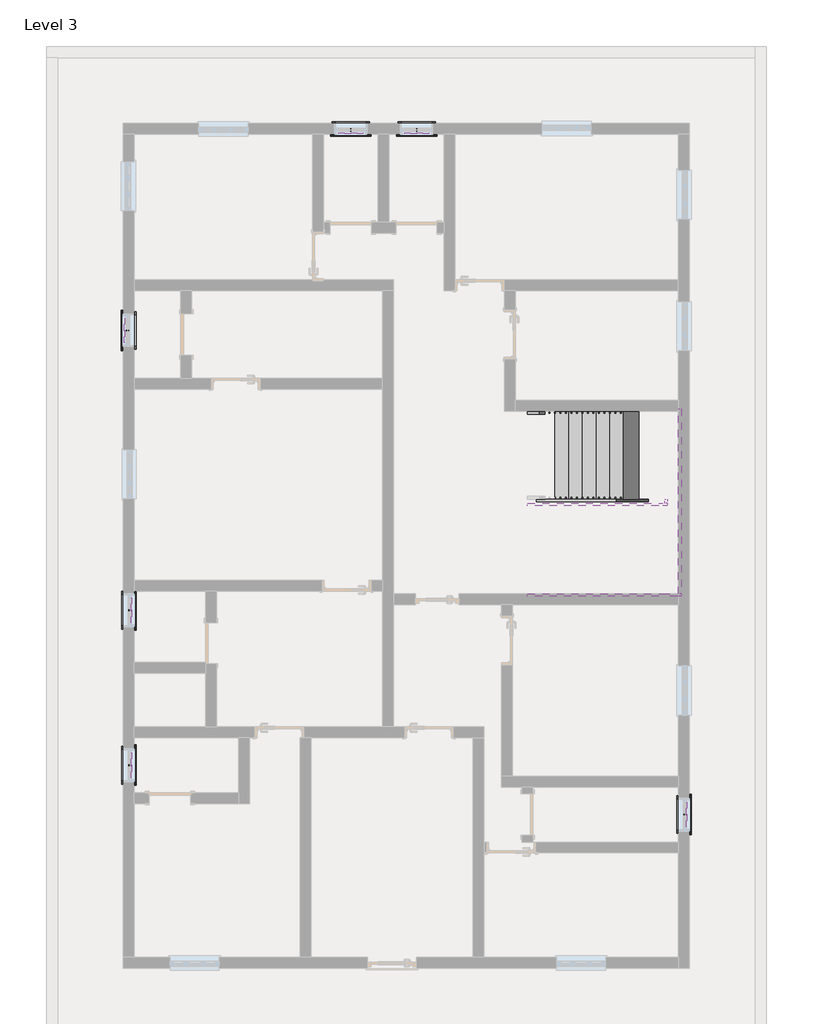
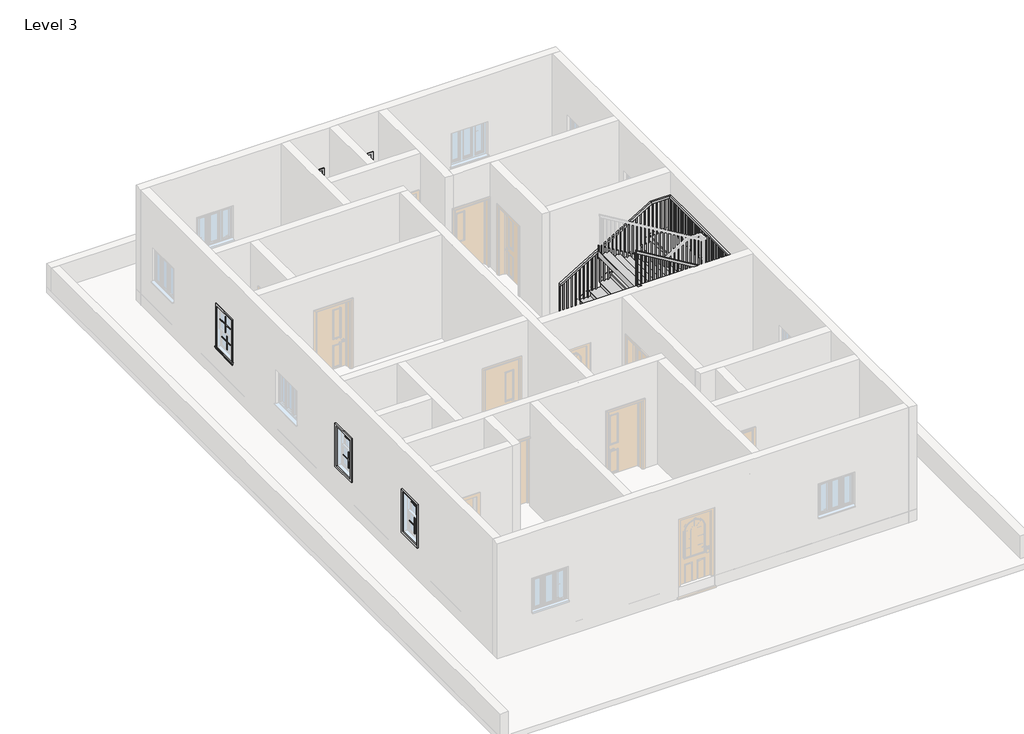
# One storey, part 3 of 3: 24 proxies, 6 members, 1 railing, 1 stair flight.
"""IFC4 building model written with IfcOpenShell, lengths in millimetres."""

from ifc_helpers import new_model, si_unit, frame, origin, place, context, project, spatial, polyline, outline, extrude, faceted_brep, transform, mapped, element, save
from components import muntin_pattern_2x2_muntin_pattern_2x2_eba6c5fb, trim_window_exterior_flat_with_sill_278e6a94, trim_window_interior_flat_picture_frame_e9fd5f45, stair_flight_8d4d0c3c

model = new_model("IFC4")

# Units and contexts
model_context = context("Model", 3, world=origin())
ifc_project = project(units=[si_unit("LENGTHUNIT", "METRE", prefix="MILLI")], contexts=[model_context])

# Site, building, storey
site = spatial("IfcSite", under=ifc_project)
building = spatial("IfcBuilding", under=site)
storey = spatial("IfcBuildingStorey", under=building, Name="Level 3", Elevation=6096.0)

# Proxies
placement = place(None, origin())
muntin_pattern_2x2_muntin_pattern_2x2_shape = muntin_pattern_2x2_muntin_pattern_2x2_eba6c5fb(model_context)
element("IfcBuildingElementProxy", 1, Name="Muntin Pattern_2x2 : Muntin Pattern_2x2", ObjectType="Muntin Pattern_2x2 : Muntin Pattern_2x2", at=placement, inside=storey, context=model_context, shape_type="MappedRepresentation", body=[
    mapped(muntin_pattern_2x2_muntin_pattern_2x2_shape, transform((-13738.8961241, 8049.5344295, 7566.025), x_axis=(0.0, -1.0, 0.0), y_axis=(1.0, 0.0, 0.0), z_axis=(0.0, 0.0, 1.0))),
])
element("IfcBuildingElementProxy", 2, Name="Muntin Pattern_2x2 : Muntin Pattern_2x2", ObjectType="Muntin Pattern_2x2 : Muntin Pattern_2x2", at=placement, inside=storey, context=model_context, shape_type="MappedRepresentation", body=[
    mapped(muntin_pattern_2x2_muntin_pattern_2x2_shape, transform((-13783.3461241, 8049.5344295, 7086.6), x_axis=(0.0, -1.0, 0.0), y_axis=(1.0, 0.0, 0.0), z_axis=(0.0, 0.0, 1.0))),
])
element("IfcBuildingElementProxy", 3, Name="Muntin Pattern_2x2 : Muntin Pattern_2x2", ObjectType="Muntin Pattern_2x2 : Muntin Pattern_2x2", at=placement, inside=storey, context=model_context, shape_type="MappedRepresentation", body=[
    mapped(muntin_pattern_2x2_muntin_pattern_2x2_shape, transform((-13738.8961241, 5179.3344295, 7566.025), x_axis=(0.0, -1.0, 0.0), y_axis=(1.0, 0.0, 0.0), z_axis=(0.0, 0.0, 1.0))),
])
element("IfcBuildingElementProxy", 4, Name="Muntin Pattern_2x2 : Muntin Pattern_2x2", ObjectType="Muntin Pattern_2x2 : Muntin Pattern_2x2", at=placement, inside=storey, context=model_context, shape_type="MappedRepresentation", body=[
    mapped(muntin_pattern_2x2_muntin_pattern_2x2_shape, transform((-13783.3461241, 5179.3344295, 7086.6), x_axis=(0.0, -1.0, 0.0), y_axis=(1.0, 0.0, 0.0), z_axis=(0.0, 0.0, 1.0))),
])
element("IfcBuildingElementProxy", 5, Name="Muntin Pattern_2x2 : Muntin Pattern_2x2", ObjectType="Muntin Pattern_2x2 : Muntin Pattern_2x2", at=placement, inside=storey, context=model_context, shape_type="MappedRepresentation", body=[
    mapped(muntin_pattern_2x2_muntin_pattern_2x2_shape, transform((-13872.2461241, 13231.1344295, 7566.025), x_axis=(0.0, 1.0, 0.0), y_axis=(-1.0, 0.0, 0.0), z_axis=(0.0, 0.0, 1.0))),
])
element("IfcBuildingElementProxy", 6, Name="Muntin Pattern_2x2 : Muntin Pattern_2x2", ObjectType="Muntin Pattern_2x2 : Muntin Pattern_2x2", at=placement, inside=storey, context=model_context, shape_type="MappedRepresentation", body=[
    mapped(muntin_pattern_2x2_muntin_pattern_2x2_shape, transform((-13827.7961241, 13231.1344295, 7086.6), x_axis=(0.0, 1.0, 0.0), y_axis=(-1.0, 0.0, 0.0), z_axis=(0.0, 0.0, 1.0))),
])
element("IfcBuildingElementProxy", 7, Name="Muntin Pattern_2x2 : Muntin Pattern_2x2", ObjectType="Muntin Pattern_2x2 : Muntin Pattern_2x2", at=placement, inside=storey, context=model_context, shape_type="MappedRepresentation", body=[
    mapped(muntin_pattern_2x2_muntin_pattern_2x2_shape, transform((-9690.7711241, 16898.2594295, 7566.025), x_axis=(-1.0, 0.0, 0.0), y_axis=(0.0, -1.0, 0.0), z_axis=(0.0, 0.0, 1.0))),
])
element("IfcBuildingElementProxy", 8, Name="Muntin Pattern_2x2 : Muntin Pattern_2x2", ObjectType="Muntin Pattern_2x2 : Muntin Pattern_2x2", at=placement, inside=storey, context=model_context, shape_type="MappedRepresentation", body=[
    mapped(muntin_pattern_2x2_muntin_pattern_2x2_shape, transform((-9690.7711241, 16942.7094295, 7086.6), x_axis=(-1.0, 0.0, 0.0), y_axis=(0.0, -1.0, 0.0), z_axis=(0.0, 0.0, 1.0))),
])
element("IfcBuildingElementProxy", 9, Name="Muntin Pattern_2x2 : Muntin Pattern_2x2", ObjectType="Muntin Pattern_2x2 : Muntin Pattern_2x2", at=placement, inside=storey, context=model_context, shape_type="MappedRepresentation", body=[
    mapped(muntin_pattern_2x2_muntin_pattern_2x2_shape, transform((-8471.5711241, 16898.2594295, 7566.025), x_axis=(-1.0, 0.0, 0.0), y_axis=(0.0, -1.0, 0.0), z_axis=(0.0, 0.0, 1.0))),
])
element("IfcBuildingElementProxy", 10, Name="Muntin Pattern_2x2 : Muntin Pattern_2x2", ObjectType="Muntin Pattern_2x2 : Muntin Pattern_2x2", at=placement, inside=storey, context=model_context, shape_type="MappedRepresentation", body=[
    mapped(muntin_pattern_2x2_muntin_pattern_2x2_shape, transform((-8471.5711241, 16942.7094295, 7086.6), x_axis=(-1.0, 0.0, 0.0), y_axis=(0.0, -1.0, 0.0), z_axis=(0.0, 0.0, 1.0))),
])
element("IfcBuildingElementProxy", 11, Name="Muntin Pattern_2x2 : Muntin Pattern_2x2", ObjectType="Muntin Pattern_2x2 : Muntin Pattern_2x2", at=placement, inside=storey, context=model_context, shape_type="MappedRepresentation", body=[
    mapped(muntin_pattern_2x2_muntin_pattern_2x2_shape, transform((-3451.8961241, 4264.9344295, 7566.025), x_axis=(0.0, -1.0, 0.0), y_axis=(1.0, 0.0, 0.0), z_axis=(0.0, 0.0, 1.0))),
])
element("IfcBuildingElementProxy", 12, Name="Muntin Pattern_2x2 : Muntin Pattern_2x2", ObjectType="Muntin Pattern_2x2 : Muntin Pattern_2x2", at=placement, inside=storey, context=model_context, shape_type="MappedRepresentation", body=[
    mapped(muntin_pattern_2x2_muntin_pattern_2x2_shape, transform((-3496.3461241, 4264.9344295, 7086.6), x_axis=(0.0, -1.0, 0.0), y_axis=(1.0, 0.0, 0.0), z_axis=(0.0, 0.0, 1.0))),
])
trim_window_exterior_flat_with_sill_shape = trim_window_exterior_flat_with_sill_278e6a94(model_context)
element("IfcBuildingElementProxy", 13, Name="Trim-Window-Exterior-Flat : with Sill", ObjectType="Trim-Window-Exterior-Flat : with Sill", at=placement, inside=storey, context=model_context, shape_type="MappedRepresentation", body=[
    mapped(trim_window_exterior_flat_with_sill_shape, transform((-13703.9711241, 8049.5344295, 8077.2), x_axis=(0.0, 1.0, 0.0), y_axis=(0.0, 0.0, 1.0), z_axis=(1.0, 0.0, 0.0))),
])
element("IfcBuildingElementProxy", 14, Name="Trim-Window-Exterior-Flat : with Sill", ObjectType="Trim-Window-Exterior-Flat : with Sill", at=placement, inside=storey, context=model_context, shape_type="MappedRepresentation", body=[
    mapped(trim_window_exterior_flat_with_sill_shape, transform((-13703.9711241, 5179.3344295, 8077.2), x_axis=(0.0, 1.0, 0.0), y_axis=(0.0, 0.0, 1.0), z_axis=(1.0, 0.0, 0.0))),
])
element("IfcBuildingElementProxy", 15, Name="Trim-Window-Exterior-Flat : with Sill", ObjectType="Trim-Window-Exterior-Flat : with Sill", at=placement, inside=storey, context=model_context, shape_type="MappedRepresentation", body=[
    mapped(trim_window_exterior_flat_with_sill_shape, transform((-13907.1711241, 13231.1344295, 8077.2), x_axis=(0.0, -1.0, 0.0), y_axis=(0.0, 0.0, 1.0), z_axis=(-1.0, 0.0, 0.0))),
])
element("IfcBuildingElementProxy", 16, Name="Trim-Window-Exterior-Flat : with Sill", ObjectType="Trim-Window-Exterior-Flat : with Sill", at=placement, inside=storey, context=model_context, shape_type="MappedRepresentation", body=[
    mapped(trim_window_exterior_flat_with_sill_shape, transform((-9690.7711241, 16863.3344295, 8077.2), x_axis=(1.0, 0.0, 0.0), y_axis=(0.0, 0.0, 1.0), z_axis=(0.0, -1.0, 0.0))),
])
element("IfcBuildingElementProxy", 17, Name="Trim-Window-Exterior-Flat : with Sill", ObjectType="Trim-Window-Exterior-Flat : with Sill", at=placement, inside=storey, context=model_context, shape_type="MappedRepresentation", body=[
    mapped(trim_window_exterior_flat_with_sill_shape, transform((-8471.5711241, 16863.3344295, 8077.2), x_axis=(1.0, 0.0, 0.0), y_axis=(0.0, 0.0, 1.0), z_axis=(0.0, -1.0, 0.0))),
])
element("IfcBuildingElementProxy", 18, Name="Trim-Window-Exterior-Flat : with Sill", ObjectType="Trim-Window-Exterior-Flat : with Sill", at=placement, inside=storey, context=model_context, shape_type="MappedRepresentation", body=[
    mapped(trim_window_exterior_flat_with_sill_shape, transform((-3416.9711241, 4264.9344295, 8077.2), x_axis=(0.0, 1.0, 0.0), y_axis=(0.0, 0.0, 1.0), z_axis=(1.0, 0.0, 0.0))),
])
trim_window_interior_flat_picture_frame_shape = trim_window_interior_flat_picture_frame_e9fd5f45(model_context)
element("IfcBuildingElementProxy", 19, Name="Trim-Window-Interior-Flat : Picture Frame", ObjectType="Trim-Window-Interior-Flat : Picture Frame", at=placement, inside=storey, context=model_context, shape_type="MappedRepresentation", body=[
    mapped(trim_window_interior_flat_picture_frame_shape, transform((-13907.1711241, 8049.5344295, 8077.2), x_axis=(0.0, -1.0, 0.0), y_axis=(0.0, 0.0, 1.0), z_axis=(-1.0, 0.0, 0.0))),
])
element("IfcBuildingElementProxy", 20, Name="Trim-Window-Interior-Flat : Picture Frame", ObjectType="Trim-Window-Interior-Flat : Picture Frame", at=placement, inside=storey, context=model_context, shape_type="MappedRepresentation", body=[
    mapped(trim_window_interior_flat_picture_frame_shape, transform((-13907.1711241, 5179.3344295, 8077.2), x_axis=(0.0, -1.0, 0.0), y_axis=(0.0, 0.0, 1.0), z_axis=(-1.0, 0.0, 0.0))),
])
element("IfcBuildingElementProxy", 21, Name="Trim-Window-Interior-Flat : Picture Frame", ObjectType="Trim-Window-Interior-Flat : Picture Frame", at=placement, inside=storey, context=model_context, shape_type="MappedRepresentation", body=[
    mapped(trim_window_interior_flat_picture_frame_shape, transform((-13703.9711241, 13231.1344295, 8077.2), x_axis=(0.0, 1.0, 0.0), y_axis=(0.0, 0.0, 1.0), z_axis=(1.0, 0.0, 0.0))),
])
element("IfcBuildingElementProxy", 22, Name="Trim-Window-Interior-Flat : Picture Frame", ObjectType="Trim-Window-Interior-Flat : Picture Frame", at=placement, inside=storey, context=model_context, shape_type="MappedRepresentation", body=[
    mapped(trim_window_interior_flat_picture_frame_shape, transform((-9690.7711241, 17066.5344295, 8077.2), x_axis=(-1.0, 0.0, 0.0), y_axis=(0.0, 0.0, 1.0), z_axis=(0.0, 1.0, 0.0))),
])
element("IfcBuildingElementProxy", 23, Name="Trim-Window-Interior-Flat : Picture Frame", ObjectType="Trim-Window-Interior-Flat : Picture Frame", at=placement, inside=storey, context=model_context, shape_type="MappedRepresentation", body=[
    mapped(trim_window_interior_flat_picture_frame_shape, transform((-8471.5711241, 17066.5344295, 8077.2), x_axis=(-1.0, 0.0, 0.0), y_axis=(0.0, 0.0, 1.0), z_axis=(0.0, 1.0, 0.0))),
])
element("IfcBuildingElementProxy", 24, Name="Trim-Window-Interior-Flat : Picture Frame", ObjectType="Trim-Window-Interior-Flat : Picture Frame", at=placement, inside=storey, context=model_context, shape_type="MappedRepresentation", body=[
    mapped(trim_window_interior_flat_picture_frame_shape, transform((-3620.1711241, 4264.9344295, 8077.2), x_axis=(0.0, -1.0, 0.0), y_axis=(0.0, 0.0, 1.0), z_axis=(-1.0, 0.0, 0.0))),
])

# Members
element("IfcMember", 25, ObjectType="Stringer - 2\" Width", at=placement, inside=storey, context=model_context, shape_type="SweptSolid", body=[
    extrude(outline(polyline([(6307.5517384, -6414.1711241), (6096.0, -6414.1711241), (6096.0, -6174.3326423), (7628.4969109, -3620.1711241), (7696.2, -3620.1711241), (7696.2, -4099.7573548), (6307.5517384, -6414.1711241)])), frame((0.0, 11732.5344295, 0.0), z_axis=(0.0, 1.0, 0.0), x_axis=(0.0, 0.0, 1.0)), (0.0, 0.0, 1.0), 50.8),
])
element("IfcMember", 26, ObjectType="Stringer - 2\" Width", at=placement, inside=storey, context=model_context, shape_type="SweptSolid", body=[
    extrude(outline(polyline([(-3620.1711241, 11783.3344295), (-3569.3711241, 11783.3344295), (-3569.3711241, 8354.3344295), (-3620.1711241, 8354.3344295), (-3620.1711241, 11783.3344295)])), frame((0.0, 0.0, 7391.4), z_axis=(0.0, 0.0, 1.0), x_axis=(1.0, 0.0, 0.0)), (0.0, 0.0, 1.0), 304.8),
])
element("IfcMember", 27, ObjectType="Stringer - 2\" Width", at=placement, inside=storey, context=model_context, shape_type="SweptSolid", body=[
    extrude(outline(polyline([(7391.4, -3569.3711241), (7496.2717384, -3569.3711241), (9203.1517384, -6414.1711241), (8847.6969109, -6414.1711241), (7391.4, -3987.0096058), (7391.4, -3569.3711241)])), frame((0.0, 8303.5344295, 0.0), z_axis=(0.0, 1.0, 0.0), x_axis=(0.0, 0.0, 1.0)), (0.0, 0.0, 1.0), 50.8),
])
element("IfcMember", 28, ObjectType="Stringer - 2\" Width", at=placement, inside=storey, context=model_context, shape_type="SweptSolid", body=[
    extrude(outline(polyline([(6307.5517384, -6414.1711241), (6096.0, -6414.1711241), (6096.0, -6174.3326423), (7476.0969109, -3874.1711241), (7696.2, -3874.1711241), (7696.2, -4099.7573548), (6307.5517384, -6414.1711241)])), frame((0.0, 10056.1344295, 0.0), z_axis=(0.0, 1.0, 0.0), x_axis=(0.0, 0.0, 1.0)), (0.0, 0.0, 1.0), 50.8),
])
element("IfcMember", 29, ObjectType="Stringer - 2\" Width", at=placement, inside=storey, context=model_context, shape_type="SweptSolid", body=[
    extrude(outline(polyline([(-3874.1711241, 10106.9344295), (-3823.3711241, 10106.9344295), (-3823.3711241, 10030.7344295), (-3874.1711241, 10030.7344295), (-3874.1711241, 10106.9344295)])), frame((0.0, 0.0, 7391.4), z_axis=(0.0, 0.0, 1.0), x_axis=(1.0, 0.0, 0.0)), (0.0, 0.0, 1.0), 304.8),
])
element("IfcMember", 30, ObjectType="Stringer - 2\" Width", at=placement, inside=storey, context=model_context, shape_type="SweptSolid", body=[
    extrude(outline(polyline([(7391.4, -3823.3711241), (7648.6717384, -3823.3711241), (9203.1517384, -6414.1711241), (8847.6969109, -6414.1711241), (7391.4, -3987.0096058), (7391.4, -3823.3711241)])), frame((0.0, 9979.9344295, 0.0), z_axis=(0.0, 1.0, 0.0), x_axis=(0.0, 0.0, 1.0)), (0.0, 0.0, 1.0), 50.8),
])

# Railing
element("IfcRailing", 31, ObjectType="Handrail - Rectangular", at=placement, inside=storey, context=model_context, shape_type="SolidModel", body=[
    faceted_brep([(-6414.1711241, 11732.5344295, 7162.8), (-6414.1711241, 11732.5344295, 7103.5575287), (-6414.1711241, 11681.7344295, 7103.5575287), (-6414.1711241, 11681.7344295, 7162.8), (-4128.1711241, 11732.5344295, 8534.4), (-4114.1003386, 11732.5344295, 8483.6), (-4114.1003386, 11681.7344295, 8483.6), (-4128.1711241, 11681.7344295, 8534.4), (-3620.1711241, 11732.5344295, 8534.4), (-3620.1711241, 11732.5344295, 8483.6), (-3670.9711241, 11681.7344295, 8483.6), (-3670.9711241, 11681.7344295, 8534.4), (-3620.1711241, 8354.3344295, 8534.4), (-3620.1711241, 8354.3344295, 8483.6), (-3670.9711241, 8405.1344295, 8483.6), (-3670.9711241, 8405.1344295, 8534.4), (-3874.1711241, 8354.3344295, 8534.4), (-3888.2419095, 8354.3344295, 8483.6), (-3888.2419095, 8405.1344295, 8483.6), (-3874.1711241, 8405.1344295, 8534.4), (-6414.1711241, 8354.3344295, 10058.4), (-6414.1711241, 8405.1344295, 10058.4), (-6414.1711241, 8405.1344295, 9999.1575287), (-6414.1711241, 8354.3344295, 9999.1575287)], [[[0, 1, 2, 3]], [[1, 0, 4, 5]], [[2, 1, 5, 6]], [[3, 2, 6, 7]], [[0, 3, 7, 4]], [[5, 4, 8, 9]], [[6, 5, 9, 10]], [[7, 6, 10, 11]], [[4, 7, 11, 8]], [[9, 8, 12, 13]], [[10, 9, 13, 14]], [[11, 10, 14, 15]], [[8, 11, 15, 12]], [[13, 12, 16, 17]], [[14, 13, 17, 18]], [[15, 14, 18, 19]], [[12, 15, 19, 16]], [[20, 21, 22, 23]], [[17, 16, 20, 23]], [[18, 17, 23, 22]], [[19, 18, 22, 21]], [[16, 19, 21, 20]]]),
    extrude(outline(polyline([(9989.6325287, -6398.2961241), (8991.6, -6398.2961241), (8991.6, -6379.2461241), (9978.2025287, -6379.2461241), (9989.6325287, -6398.2961241)])), frame((0.0, 8370.2094295, 0.0), z_axis=(0.0, 1.0, 0.0), x_axis=(0.0, 0.0, 1.0)), (0.0, 0.0, 1.0), 19.05),
    extrude(outline(polyline([(9928.6725287, -6296.6961241), (8991.6, -6296.6961241), (8991.6, -6277.6461241), (9917.2425287, -6277.6461241), (9928.6725287, -6296.6961241)])), frame((0.0, 8370.2094295, 0.0), z_axis=(0.0, 1.0, 0.0), x_axis=(0.0, 0.0, 1.0)), (0.0, 0.0, 1.0), 19.05),
    extrude(outline(polyline([(9867.7125287, -6195.0961241), (8991.6, -6195.0961241), (8991.6, -6176.0461241), (9856.2825287, -6176.0461241), (9867.7125287, -6195.0961241)])), frame((0.0, 8370.2094295, 0.0), z_axis=(0.0, 1.0, 0.0), x_axis=(0.0, 0.0, 1.0)), (0.0, 0.0, 1.0), 19.05),
    extrude(outline(polyline([(9806.7525287, -6093.4961241), (8839.2, -6093.4961241), (8839.2, -6074.4461241), (9795.3225287, -6074.4461241), (9806.7525287, -6093.4961241)])), frame((0.0, 8370.2094295, 0.0), z_axis=(0.0, 1.0, 0.0), x_axis=(0.0, 0.0, 1.0)), (0.0, 0.0, 1.0), 19.05),
    extrude(outline(polyline([(9745.7925287, -5991.8961241), (8839.2, -5991.8961241), (8839.2, -5972.8461241), (9734.3625287, -5972.8461241), (9745.7925287, -5991.8961241)])), frame((0.0, 8370.2094295, 0.0), z_axis=(0.0, 1.0, 0.0), x_axis=(0.0, 0.0, 1.0)), (0.0, 0.0, 1.0), 19.05),
    extrude(outline(polyline([(9684.8325287, -5890.2961241), (8686.8, -5890.2961241), (8686.8, -5871.2461241), (9673.4025287, -5871.2461241), (9684.8325287, -5890.2961241)])), frame((0.0, 8370.2094295, 0.0), z_axis=(0.0, 1.0, 0.0), x_axis=(0.0, 0.0, 1.0)), (0.0, 0.0, 1.0), 19.05),
    extrude(outline(polyline([(9623.8725287, -5788.6961241), (8686.8, -5788.6961241), (8686.8, -5769.6461241), (9612.4425287, -5769.6461241), (9623.8725287, -5788.6961241)])), frame((0.0, 8370.2094295, 0.0), z_axis=(0.0, 1.0, 0.0), x_axis=(0.0, 0.0, 1.0)), (0.0, 0.0, 1.0), 19.05),
    extrude(outline(polyline([(9562.9125287, -5687.0961241), (8686.8, -5687.0961241), (8686.8, -5668.0461241), (9551.4825287, -5668.0461241), (9562.9125287, -5687.0961241)])), frame((0.0, 8370.2094295, 0.0), z_axis=(0.0, 1.0, 0.0), x_axis=(0.0, 0.0, 1.0)), (0.0, 0.0, 1.0), 19.05),
    extrude(outline(polyline([(9501.9525287, -5585.4961241), (8534.4, -5585.4961241), (8534.4, -5566.4461241), (9490.5225287, -5566.4461241), (9501.9525287, -5585.4961241)])), frame((0.0, 8370.2094295, 0.0), z_axis=(0.0, 1.0, 0.0), x_axis=(0.0, 0.0, 1.0)), (0.0, 0.0, 1.0), 19.05),
    extrude(outline(polyline([(9440.9925287, -5483.8961241), (8534.4, -5483.8961241), (8534.4, -5464.8461241), (9429.5625287, -5464.8461241), (9440.9925287, -5483.8961241)])), frame((0.0, 8370.2094295, 0.0), z_axis=(0.0, 1.0, 0.0), x_axis=(0.0, 0.0, 1.0)), (0.0, 0.0, 1.0), 19.05),
    extrude(outline(polyline([(9380.0325287, -5382.2961241), (8382.0, -5382.2961241), (8382.0, -5363.2461241), (9368.6025287, -5363.2461241), (9380.0325287, -5382.2961241)])), frame((0.0, 8370.2094295, 0.0), z_axis=(0.0, 1.0, 0.0), x_axis=(0.0, 0.0, 1.0)), (0.0, 0.0, 1.0), 19.05),
    extrude(outline(polyline([(9319.0725287, -5280.6961241), (8382.0, -5280.6961241), (8382.0, -5261.6461241), (9307.6425287, -5261.6461241), (9319.0725287, -5280.6961241)])), frame((0.0, 8370.2094295, 0.0), z_axis=(0.0, 1.0, 0.0), x_axis=(0.0, 0.0, 1.0)), (0.0, 0.0, 1.0), 19.05),
    extrude(outline(polyline([(9258.1125287, -5179.0961241), (8382.0, -5179.0961241), (8382.0, -5160.0461241), (9246.6825287, -5160.0461241), (9258.1125287, -5179.0961241)])), frame((0.0, 8370.2094295, 0.0), z_axis=(0.0, 1.0, 0.0), x_axis=(0.0, 0.0, 1.0)), (0.0, 0.0, 1.0), 19.05),
    extrude(outline(polyline([(9197.1525287, -5077.4961241), (8229.6, -5077.4961241), (8229.6, -5058.4461241), (9185.7225287, -5058.4461241), (9197.1525287, -5077.4961241)])), frame((0.0, 8370.2094295, 0.0), z_axis=(0.0, 1.0, 0.0), x_axis=(0.0, 0.0, 1.0)), (0.0, 0.0, 1.0), 19.05),
    extrude(outline(polyline([(9136.1925287, -4975.8961241), (8229.6, -4975.8961241), (8229.6, -4956.8461241), (9124.7625287, -4956.8461241), (9136.1925287, -4975.8961241)])), frame((0.0, 8370.2094295, 0.0), z_axis=(0.0, 1.0, 0.0), x_axis=(0.0, 0.0, 1.0)), (0.0, 0.0, 1.0), 19.05),
    extrude(outline(polyline([(9075.2325287, -4874.2961241), (8077.2, -4874.2961241), (8077.2, -4855.2461241), (9063.8025287, -4855.2461241), (9075.2325287, -4874.2961241)])), frame((0.0, 8370.2094295, 0.0), z_axis=(0.0, 1.0, 0.0), x_axis=(0.0, 0.0, 1.0)), (0.0, 0.0, 1.0), 19.05),
    extrude(outline(polyline([(9014.2725287, -4772.6961241), (8077.2, -4772.6961241), (8077.2, -4753.6461241), (9002.8425287, -4753.6461241), (9014.2725287, -4772.6961241)])), frame((0.0, 8370.2094295, 0.0), z_axis=(0.0, 1.0, 0.0), x_axis=(0.0, 0.0, 1.0)), (0.0, 0.0, 1.0), 19.05),
    extrude(outline(polyline([(8953.3125287, -4671.0961241), (8077.2, -4671.0961241), (8077.2, -4652.0461241), (8941.8825287, -4652.0461241), (8953.3125287, -4671.0961241)])), frame((0.0, 8370.2094295, 0.0), z_axis=(0.0, 1.0, 0.0), x_axis=(0.0, 0.0, 1.0)), (0.0, 0.0, 1.0), 19.05),
    extrude(outline(polyline([(8892.3525287, -4569.4961241), (7924.8, -4569.4961241), (7924.8, -4550.4461241), (8880.9225287, -4550.4461241), (8892.3525287, -4569.4961241)])), frame((0.0, 8370.2094295, 0.0), z_axis=(0.0, 1.0, 0.0), x_axis=(0.0, 0.0, 1.0)), (0.0, 0.0, 1.0), 19.05),
    extrude(outline(polyline([(8831.3925287, -4467.8961241), (7924.8, -4467.8961241), (7924.8, -4448.8461241), (8819.9625287, -4448.8461241), (8831.3925287, -4467.8961241)])), frame((0.0, 8370.2094295, 0.0), z_axis=(0.0, 1.0, 0.0), x_axis=(0.0, 0.0, 1.0)), (0.0, 0.0, 1.0), 19.05),
    extrude(outline(polyline([(8770.4325287, -4366.2961241), (7772.4, -4366.2961241), (7772.4, -4347.2461241), (8759.0025287, -4347.2461241), (8770.4325287, -4366.2961241)])), frame((0.0, 8370.2094295, 0.0), z_axis=(0.0, 1.0, 0.0), x_axis=(0.0, 0.0, 1.0)), (0.0, 0.0, 1.0), 19.05),
    extrude(outline(polyline([(8709.4725287, -4264.6961241), (7772.4, -4264.6961241), (7772.4, -4245.6461241), (8698.0425287, -4245.6461241), (8709.4725287, -4264.6961241)])), frame((0.0, 8370.2094295, 0.0), z_axis=(0.0, 1.0, 0.0), x_axis=(0.0, 0.0, 1.0)), (0.0, 0.0, 1.0), 19.05),
    extrude(outline(polyline([(8648.5125287, -4163.0961241), (7772.4, -4163.0961241), (7772.4, -4144.0461241), (8637.0825287, -4144.0461241), (8648.5125287, -4163.0961241)])), frame((0.0, 8370.2094295, 0.0), z_axis=(0.0, 1.0, 0.0), x_axis=(0.0, 0.0, 1.0)), (0.0, 0.0, 1.0), 19.05),
    extrude(outline(polyline([(8587.5525287, -4061.4961241), (7620.0, -4061.4961241), (7620.0, -4042.4461241), (8576.1225287, -4042.4461241), (8587.5525287, -4061.4961241)])), frame((0.0, 8370.2094295, 0.0), z_axis=(0.0, 1.0, 0.0), x_axis=(0.0, 0.0, 1.0)), (0.0, 0.0, 1.0), 19.05),
    extrude(outline(polyline([(8526.5925287, -3959.8961241), (7620.0, -3959.8961241), (7620.0, -3940.8461241), (8515.1625287, -3940.8461241), (8526.5925287, -3959.8961241)])), frame((0.0, 8370.2094295, 0.0), z_axis=(0.0, 1.0, 0.0), x_axis=(0.0, 0.0, 1.0)), (0.0, 0.0, 1.0), 19.05),
    extrude(outline(polyline([(-3839.2461241, 8370.2094295), (-3858.2961241, 8370.2094295), (-3858.2961241, 8389.2594295), (-3839.2461241, 8389.2594295), (-3839.2461241, 8370.2094295)])), frame((0.0, 0.0, 7620.0), z_axis=(0.0, 0.0, 1.0), x_axis=(1.0, 0.0, 0.0)), (0.0, 0.0, 1.0), 863.6),
    extrude(outline(polyline([(-3737.6461241, 8370.2094295), (-3756.6961241, 8370.2094295), (-3756.6961241, 8389.2594295), (-3737.6461241, 8389.2594295), (-3737.6461241, 8370.2094295)])), frame((0.0, 0.0, 7620.0), z_axis=(0.0, 0.0, 1.0), x_axis=(1.0, 0.0, 0.0)), (0.0, 0.0, 1.0), 863.6),
    extrude(outline(polyline([(-3636.0461241, 8465.4594295), (-3636.0461241, 8446.4094295), (-3655.0961241, 8446.4094295), (-3655.0961241, 8465.4594295), (-3636.0461241, 8465.4594295)])), frame((0.0, 0.0, 7620.0), z_axis=(0.0, 0.0, 1.0), x_axis=(1.0, 0.0, 0.0)), (0.0, 0.0, 1.0), 863.6),
    extrude(outline(polyline([(-3636.0461241, 8567.0594295), (-3636.0461241, 8548.0094295), (-3655.0961241, 8548.0094295), (-3655.0961241, 8567.0594295), (-3636.0461241, 8567.0594295)])), frame((0.0, 0.0, 7620.0), z_axis=(0.0, 0.0, 1.0), x_axis=(1.0, 0.0, 0.0)), (0.0, 0.0, 1.0), 863.6),
    extrude(outline(polyline([(-3636.0461241, 8668.6594295), (-3636.0461241, 8649.6094295), (-3655.0961241, 8649.6094295), (-3655.0961241, 8668.6594295), (-3636.0461241, 8668.6594295)])), frame((0.0, 0.0, 7620.0), z_axis=(0.0, 0.0, 1.0), x_axis=(1.0, 0.0, 0.0)), (0.0, 0.0, 1.0), 863.6),
    extrude(outline(polyline([(-3636.0461241, 8770.2594295), (-3636.0461241, 8751.2094295), (-3655.0961241, 8751.2094295), (-3655.0961241, 8770.2594295), (-3636.0461241, 8770.2594295)])), frame((0.0, 0.0, 7620.0), z_axis=(0.0, 0.0, 1.0), x_axis=(1.0, 0.0, 0.0)), (0.0, 0.0, 1.0), 863.6),
    extrude(outline(polyline([(-3636.0461241, 8871.8594295), (-3636.0461241, 8852.8094295), (-3655.0961241, 8852.8094295), (-3655.0961241, 8871.8594295), (-3636.0461241, 8871.8594295)])), frame((0.0, 0.0, 7620.0), z_axis=(0.0, 0.0, 1.0), x_axis=(1.0, 0.0, 0.0)), (0.0, 0.0, 1.0), 863.6),
    extrude(outline(polyline([(-3636.0461241, 8973.4594295), (-3636.0461241, 8954.4094295), (-3655.0961241, 8954.4094295), (-3655.0961241, 8973.4594295), (-3636.0461241, 8973.4594295)])), frame((0.0, 0.0, 7620.0), z_axis=(0.0, 0.0, 1.0), x_axis=(1.0, 0.0, 0.0)), (0.0, 0.0, 1.0), 863.6),
    extrude(outline(polyline([(-3636.0461241, 9075.0594295), (-3636.0461241, 9056.0094295), (-3655.0961241, 9056.0094295), (-3655.0961241, 9075.0594295), (-3636.0461241, 9075.0594295)])), frame((0.0, 0.0, 7620.0), z_axis=(0.0, 0.0, 1.0), x_axis=(1.0, 0.0, 0.0)), (0.0, 0.0, 1.0), 863.6),
    extrude(outline(polyline([(-3636.0461241, 9176.6594295), (-3636.0461241, 9157.6094295), (-3655.0961241, 9157.6094295), (-3655.0961241, 9176.6594295), (-3636.0461241, 9176.6594295)])), frame((0.0, 0.0, 7620.0), z_axis=(0.0, 0.0, 1.0), x_axis=(1.0, 0.0, 0.0)), (0.0, 0.0, 1.0), 863.6),
    extrude(outline(polyline([(-3636.0461241, 9278.2594295), (-3636.0461241, 9259.2094295), (-3655.0961241, 9259.2094295), (-3655.0961241, 9278.2594295), (-3636.0461241, 9278.2594295)])), frame((0.0, 0.0, 7620.0), z_axis=(0.0, 0.0, 1.0), x_axis=(1.0, 0.0, 0.0)), (0.0, 0.0, 1.0), 863.6),
    extrude(outline(polyline([(-3636.0461241, 9379.8594295), (-3636.0461241, 9360.8094295), (-3655.0961241, 9360.8094295), (-3655.0961241, 9379.8594295), (-3636.0461241, 9379.8594295)])), frame((0.0, 0.0, 7620.0), z_axis=(0.0, 0.0, 1.0), x_axis=(1.0, 0.0, 0.0)), (0.0, 0.0, 1.0), 863.6),
    extrude(outline(polyline([(-3636.0461241, 9481.4594295), (-3636.0461241, 9462.4094295), (-3655.0961241, 9462.4094295), (-3655.0961241, 9481.4594295), (-3636.0461241, 9481.4594295)])), frame((0.0, 0.0, 7620.0), z_axis=(0.0, 0.0, 1.0), x_axis=(1.0, 0.0, 0.0)), (0.0, 0.0, 1.0), 863.6),
    extrude(outline(polyline([(-3636.0461241, 9583.0594295), (-3636.0461241, 9564.0094295), (-3655.0961241, 9564.0094295), (-3655.0961241, 9583.0594295), (-3636.0461241, 9583.0594295)])), frame((0.0, 0.0, 7620.0), z_axis=(0.0, 0.0, 1.0), x_axis=(1.0, 0.0, 0.0)), (0.0, 0.0, 1.0), 863.6),
    extrude(outline(polyline([(-3636.0461241, 9684.6594295), (-3636.0461241, 9665.6094295), (-3655.0961241, 9665.6094295), (-3655.0961241, 9684.6594295), (-3636.0461241, 9684.6594295)])), frame((0.0, 0.0, 7620.0), z_axis=(0.0, 0.0, 1.0), x_axis=(1.0, 0.0, 0.0)), (0.0, 0.0, 1.0), 863.6),
    extrude(outline(polyline([(-3636.0461241, 9786.2594295), (-3636.0461241, 9767.2094295), (-3655.0961241, 9767.2094295), (-3655.0961241, 9786.2594295), (-3636.0461241, 9786.2594295)])), frame((0.0, 0.0, 7620.0), z_axis=(0.0, 0.0, 1.0), x_axis=(1.0, 0.0, 0.0)), (0.0, 0.0, 1.0), 863.6),
    extrude(outline(polyline([(-3636.0461241, 9887.8594295), (-3636.0461241, 9868.8094295), (-3655.0961241, 9868.8094295), (-3655.0961241, 9887.8594295), (-3636.0461241, 9887.8594295)])), frame((0.0, 0.0, 7620.0), z_axis=(0.0, 0.0, 1.0), x_axis=(1.0, 0.0, 0.0)), (0.0, 0.0, 1.0), 863.6),
    extrude(outline(polyline([(-3636.0461241, 9989.4594295), (-3636.0461241, 9970.4094295), (-3655.0961241, 9970.4094295), (-3655.0961241, 9989.4594295), (-3636.0461241, 9989.4594295)])), frame((0.0, 0.0, 7620.0), z_axis=(0.0, 0.0, 1.0), x_axis=(1.0, 0.0, 0.0)), (0.0, 0.0, 1.0), 863.6),
    extrude(outline(polyline([(-3636.0461241, 10091.0594295), (-3636.0461241, 10072.0094295), (-3655.0961241, 10072.0094295), (-3655.0961241, 10091.0594295), (-3636.0461241, 10091.0594295)])), frame((0.0, 0.0, 7620.0), z_axis=(0.0, 0.0, 1.0), x_axis=(1.0, 0.0, 0.0)), (0.0, 0.0, 1.0), 863.6),
    extrude(outline(polyline([(-3636.0461241, 10192.6594295), (-3636.0461241, 10173.6094295), (-3655.0961241, 10173.6094295), (-3655.0961241, 10192.6594295), (-3636.0461241, 10192.6594295)])), frame((0.0, 0.0, 7620.0), z_axis=(0.0, 0.0, 1.0), x_axis=(1.0, 0.0, 0.0)), (0.0, 0.0, 1.0), 863.6),
    extrude(outline(polyline([(-3636.0461241, 10294.2594295), (-3636.0461241, 10275.2094295), (-3655.0961241, 10275.2094295), (-3655.0961241, 10294.2594295), (-3636.0461241, 10294.2594295)])), frame((0.0, 0.0, 7620.0), z_axis=(0.0, 0.0, 1.0), x_axis=(1.0, 0.0, 0.0)), (0.0, 0.0, 1.0), 863.6),
    extrude(outline(polyline([(-3636.0461241, 10395.8594295), (-3636.0461241, 10376.8094295), (-3655.0961241, 10376.8094295), (-3655.0961241, 10395.8594295), (-3636.0461241, 10395.8594295)])), frame((0.0, 0.0, 7620.0), z_axis=(0.0, 0.0, 1.0), x_axis=(1.0, 0.0, 0.0)), (0.0, 0.0, 1.0), 863.6),
    extrude(outline(polyline([(-3636.0461241, 10497.4594295), (-3636.0461241, 10478.4094295), (-3655.0961241, 10478.4094295), (-3655.0961241, 10497.4594295), (-3636.0461241, 10497.4594295)])), frame((0.0, 0.0, 7620.0), z_axis=(0.0, 0.0, 1.0), x_axis=(1.0, 0.0, 0.0)), (0.0, 0.0, 1.0), 863.6),
    extrude(outline(polyline([(-3636.0461241, 10599.0594295), (-3636.0461241, 10580.0094295), (-3655.0961241, 10580.0094295), (-3655.0961241, 10599.0594295), (-3636.0461241, 10599.0594295)])), frame((0.0, 0.0, 7620.0), z_axis=(0.0, 0.0, 1.0), x_axis=(1.0, 0.0, 0.0)), (0.0, 0.0, 1.0), 863.6),
    extrude(outline(polyline([(-3636.0461241, 10700.6594295), (-3636.0461241, 10681.6094295), (-3655.0961241, 10681.6094295), (-3655.0961241, 10700.6594295), (-3636.0461241, 10700.6594295)])), frame((0.0, 0.0, 7620.0), z_axis=(0.0, 0.0, 1.0), x_axis=(1.0, 0.0, 0.0)), (0.0, 0.0, 1.0), 863.6),
    extrude(outline(polyline([(-3636.0461241, 10802.2594295), (-3636.0461241, 10783.2094295), (-3655.0961241, 10783.2094295), (-3655.0961241, 10802.2594295), (-3636.0461241, 10802.2594295)])), frame((0.0, 0.0, 7620.0), z_axis=(0.0, 0.0, 1.0), x_axis=(1.0, 0.0, 0.0)), (0.0, 0.0, 1.0), 863.6),
    extrude(outline(polyline([(-3636.0461241, 10903.8594295), (-3636.0461241, 10884.8094295), (-3655.0961241, 10884.8094295), (-3655.0961241, 10903.8594295), (-3636.0461241, 10903.8594295)])), frame((0.0, 0.0, 7620.0), z_axis=(0.0, 0.0, 1.0), x_axis=(1.0, 0.0, 0.0)), (0.0, 0.0, 1.0), 863.6),
    extrude(outline(polyline([(-3636.0461241, 11005.4594295), (-3636.0461241, 10986.4094295), (-3655.0961241, 10986.4094295), (-3655.0961241, 11005.4594295), (-3636.0461241, 11005.4594295)])), frame((0.0, 0.0, 7620.0), z_axis=(0.0, 0.0, 1.0), x_axis=(1.0, 0.0, 0.0)), (0.0, 0.0, 1.0), 863.6),
    extrude(outline(polyline([(-3636.0461241, 11107.0594295), (-3636.0461241, 11088.0094295), (-3655.0961241, 11088.0094295), (-3655.0961241, 11107.0594295), (-3636.0461241, 11107.0594295)])), frame((0.0, 0.0, 7620.0), z_axis=(0.0, 0.0, 1.0), x_axis=(1.0, 0.0, 0.0)), (0.0, 0.0, 1.0), 863.6),
    extrude(outline(polyline([(-3636.0461241, 11208.6594295), (-3636.0461241, 11189.6094295), (-3655.0961241, 11189.6094295), (-3655.0961241, 11208.6594295), (-3636.0461241, 11208.6594295)])), frame((0.0, 0.0, 7620.0), z_axis=(0.0, 0.0, 1.0), x_axis=(1.0, 0.0, 0.0)), (0.0, 0.0, 1.0), 863.6),
    extrude(outline(polyline([(-3636.0461241, 11310.2594295), (-3636.0461241, 11291.2094295), (-3655.0961241, 11291.2094295), (-3655.0961241, 11310.2594295), (-3636.0461241, 11310.2594295)])), frame((0.0, 0.0, 7620.0), z_axis=(0.0, 0.0, 1.0), x_axis=(1.0, 0.0, 0.0)), (0.0, 0.0, 1.0), 863.6),
    extrude(outline(polyline([(-3636.0461241, 11411.8594295), (-3636.0461241, 11392.8094295), (-3655.0961241, 11392.8094295), (-3655.0961241, 11411.8594295), (-3636.0461241, 11411.8594295)])), frame((0.0, 0.0, 7620.0), z_axis=(0.0, 0.0, 1.0), x_axis=(1.0, 0.0, 0.0)), (0.0, 0.0, 1.0), 863.6),
    extrude(outline(polyline([(-3636.0461241, 11513.4594295), (-3636.0461241, 11494.4094295), (-3655.0961241, 11494.4094295), (-3655.0961241, 11513.4594295), (-3636.0461241, 11513.4594295)])), frame((0.0, 0.0, 7620.0), z_axis=(0.0, 0.0, 1.0), x_axis=(1.0, 0.0, 0.0)), (0.0, 0.0, 1.0), 863.6),
    extrude(outline(polyline([(-3636.0461241, 11615.0594295), (-3636.0461241, 11596.0094295), (-3655.0961241, 11596.0094295), (-3655.0961241, 11615.0594295), (-3636.0461241, 11615.0594295)])), frame((0.0, 0.0, 7620.0), z_axis=(0.0, 0.0, 1.0), x_axis=(1.0, 0.0, 0.0)), (0.0, 0.0, 1.0), 863.6),
    extrude(outline(polyline([(-3680.4961241, 11716.6594295), (-3661.4461241, 11716.6594295), (-3661.4461241, 11697.6094295), (-3680.4961241, 11697.6094295), (-3680.4961241, 11716.6594295)])), frame((0.0, 0.0, 7620.0), z_axis=(0.0, 0.0, 1.0), x_axis=(1.0, 0.0, 0.0)), (0.0, 0.0, 1.0), 863.6),
    extrude(outline(polyline([(-3782.0961241, 11716.6594295), (-3763.0461241, 11716.6594295), (-3763.0461241, 11697.6094295), (-3782.0961241, 11697.6094295), (-3782.0961241, 11716.6594295)])), frame((0.0, 0.0, 7620.0), z_axis=(0.0, 0.0, 1.0), x_axis=(1.0, 0.0, 0.0)), (0.0, 0.0, 1.0), 863.6),
    extrude(outline(polyline([(-3883.6961241, 11716.6594295), (-3864.6461241, 11716.6594295), (-3864.6461241, 11697.6094295), (-3883.6961241, 11697.6094295), (-3883.6961241, 11716.6594295)])), frame((0.0, 0.0, 7620.0), z_axis=(0.0, 0.0, 1.0), x_axis=(1.0, 0.0, 0.0)), (0.0, 0.0, 1.0), 863.6),
    extrude(outline(polyline([(-3985.2961241, 11716.6594295), (-3966.2461241, 11716.6594295), (-3966.2461241, 11697.6094295), (-3985.2961241, 11697.6094295), (-3985.2961241, 11716.6594295)])), frame((0.0, 0.0, 7620.0), z_axis=(0.0, 0.0, 1.0), x_axis=(1.0, 0.0, 0.0)), (0.0, 0.0, 1.0), 863.6),
    extrude(outline(polyline([(-4086.8961241, 11716.6594295), (-4067.8461241, 11716.6594295), (-4067.8461241, 11697.6094295), (-4086.8961241, 11697.6094295), (-4086.8961241, 11716.6594295)])), frame((0.0, 0.0, 7620.0), z_axis=(0.0, 0.0, 1.0), x_axis=(1.0, 0.0, 0.0)), (0.0, 0.0, 1.0), 863.6),
    extrude(outline(polyline([(8438.9625287, -4188.4961241), (7467.6, -4188.4961241), (7467.6, -4169.4461241), (8450.3925287, -4169.4461241), (8438.9625287, -4188.4961241)])), frame((0.0, 11697.6094295, 0.0), z_axis=(0.0, 1.0, 0.0), x_axis=(0.0, 0.0, 1.0)), (0.0, 0.0, 1.0), 19.05),
    extrude(outline(polyline([(8378.0025287, -4290.0961241), (7467.6, -4290.0961241), (7467.6, -4271.0461241), (8389.4325287, -4271.0461241), (8378.0025287, -4290.0961241)])), frame((0.0, 11697.6094295, 0.0), z_axis=(0.0, 1.0, 0.0), x_axis=(0.0, 0.0, 1.0)), (0.0, 0.0, 1.0), 19.05),
    extrude(outline(polyline([(8317.0425287, -4391.6961241), (7467.6, -4391.6961241), (7467.6, -4372.6461241), (8328.4725287, -4372.6461241), (8317.0425287, -4391.6961241)])), frame((0.0, 11697.6094295, 0.0), z_axis=(0.0, 1.0, 0.0), x_axis=(0.0, 0.0, 1.0)), (0.0, 0.0, 1.0), 19.05),
    extrude(outline(polyline([(8256.0825287, -4493.2961241), (7315.2, -4493.2961241), (7315.2, -4474.2461241), (8267.5125287, -4474.2461241), (8256.0825287, -4493.2961241)])), frame((0.0, 11697.6094295, 0.0), z_axis=(0.0, 1.0, 0.0), x_axis=(0.0, 0.0, 1.0)), (0.0, 0.0, 1.0), 19.05),
    extrude(outline(polyline([(8195.1225287, -4594.8961241), (7315.2, -4594.8961241), (7315.2, -4575.8461241), (8206.5525287, -4575.8461241), (8195.1225287, -4594.8961241)])), frame((0.0, 11697.6094295, 0.0), z_axis=(0.0, 1.0, 0.0), x_axis=(0.0, 0.0, 1.0)), (0.0, 0.0, 1.0), 19.05),
    extrude(outline(polyline([(8134.1625287, -4696.4961241), (7162.8, -4696.4961241), (7162.8, -4677.4461241), (8145.5925287, -4677.4461241), (8134.1625287, -4696.4961241)])), frame((0.0, 11697.6094295, 0.0), z_axis=(0.0, 1.0, 0.0), x_axis=(0.0, 0.0, 1.0)), (0.0, 0.0, 1.0), 19.05),
    extrude(outline(polyline([(8073.2025287, -4798.0961241), (7162.8, -4798.0961241), (7162.8, -4779.0461241), (8084.6325287, -4779.0461241), (8073.2025287, -4798.0961241)])), frame((0.0, 11697.6094295, 0.0), z_axis=(0.0, 1.0, 0.0), x_axis=(0.0, 0.0, 1.0)), (0.0, 0.0, 1.0), 19.05),
    extrude(outline(polyline([(8012.2425287, -4899.6961241), (7162.8, -4899.6961241), (7162.8, -4880.6461241), (8023.6725287, -4880.6461241), (8012.2425287, -4899.6961241)])), frame((0.0, 11697.6094295, 0.0), z_axis=(0.0, 1.0, 0.0), x_axis=(0.0, 0.0, 1.0)), (0.0, 0.0, 1.0), 19.05),
    extrude(outline(polyline([(7951.2825287, -5001.2961241), (7010.4, -5001.2961241), (7010.4, -4982.2461241), (7962.7125287, -4982.2461241), (7951.2825287, -5001.2961241)])), frame((0.0, 11697.6094295, 0.0), z_axis=(0.0, 1.0, 0.0), x_axis=(0.0, 0.0, 1.0)), (0.0, 0.0, 1.0), 19.05),
    extrude(outline(polyline([(7890.3225287, -5102.8961241), (7010.4, -5102.8961241), (7010.4, -5083.8461241), (7901.7525287, -5083.8461241), (7890.3225287, -5102.8961241)])), frame((0.0, 11697.6094295, 0.0), z_axis=(0.0, 1.0, 0.0), x_axis=(0.0, 0.0, 1.0)), (0.0, 0.0, 1.0), 19.05),
    extrude(outline(polyline([(7829.3625287, -5204.4961241), (6858.0, -5204.4961241), (6858.0, -5185.4461241), (7840.7925287, -5185.4461241), (7829.3625287, -5204.4961241)])), frame((0.0, 11697.6094295, 0.0), z_axis=(0.0, 1.0, 0.0), x_axis=(0.0, 0.0, 1.0)), (0.0, 0.0, 1.0), 19.05),
    extrude(outline(polyline([(7768.4025287, -5306.0961241), (6858.0, -5306.0961241), (6858.0, -5287.0461241), (7779.8325287, -5287.0461241), (7768.4025287, -5306.0961241)])), frame((0.0, 11697.6094295, 0.0), z_axis=(0.0, 1.0, 0.0), x_axis=(0.0, 0.0, 1.0)), (0.0, 0.0, 1.0), 19.05),
    extrude(outline(polyline([(7707.4425287, -5407.6961241), (6858.0, -5407.6961241), (6858.0, -5388.6461241), (7718.8725287, -5388.6461241), (7707.4425287, -5407.6961241)])), frame((0.0, 11697.6094295, 0.0), z_axis=(0.0, 1.0, 0.0), x_axis=(0.0, 0.0, 1.0)), (0.0, 0.0, 1.0), 19.05),
    extrude(outline(polyline([(7646.4825287, -5509.2961241), (6705.6, -5509.2961241), (6705.6, -5490.2461241), (7657.9125287, -5490.2461241), (7646.4825287, -5509.2961241)])), frame((0.0, 11697.6094295, 0.0), z_axis=(0.0, 1.0, 0.0), x_axis=(0.0, 0.0, 1.0)), (0.0, 0.0, 1.0), 19.05),
    extrude(outline(polyline([(7585.5225287, -5610.8961241), (6705.6, -5610.8961241), (6705.6, -5591.8461241), (7596.9525287, -5591.8461241), (7585.5225287, -5610.8961241)])), frame((0.0, 11697.6094295, 0.0), z_axis=(0.0, 1.0, 0.0), x_axis=(0.0, 0.0, 1.0)), (0.0, 0.0, 1.0), 19.05),
    extrude(outline(polyline([(7524.5625287, -5712.4961241), (6553.2, -5712.4961241), (6553.2, -5693.4461241), (7535.9925287, -5693.4461241), (7524.5625287, -5712.4961241)])), frame((0.0, 11697.6094295, 0.0), z_axis=(0.0, 1.0, 0.0), x_axis=(0.0, 0.0, 1.0)), (0.0, 0.0, 1.0), 19.05),
    extrude(outline(polyline([(7463.6025287, -5814.0961241), (6553.2, -5814.0961241), (6553.2, -5795.0461241), (7475.0325287, -5795.0461241), (7463.6025287, -5814.0961241)])), frame((0.0, 11697.6094295, 0.0), z_axis=(0.0, 1.0, 0.0), x_axis=(0.0, 0.0, 1.0)), (0.0, 0.0, 1.0), 19.05),
    extrude(outline(polyline([(7402.6425287, -5915.6961241), (6553.2, -5915.6961241), (6553.2, -5896.6461241), (7414.0725287, -5896.6461241), (7402.6425287, -5915.6961241)])), frame((0.0, 11697.6094295, 0.0), z_axis=(0.0, 1.0, 0.0), x_axis=(0.0, 0.0, 1.0)), (0.0, 0.0, 1.0), 19.05),
    extrude(outline(polyline([(7341.6825287, -6017.2961241), (6400.8, -6017.2961241), (6400.8, -5998.2461241), (7353.1125287, -5998.2461241), (7341.6825287, -6017.2961241)])), frame((0.0, 11697.6094295, 0.0), z_axis=(0.0, 1.0, 0.0), x_axis=(0.0, 0.0, 1.0)), (0.0, 0.0, 1.0), 19.05),
    extrude(outline(polyline([(7280.7225287, -6118.8961241), (6400.8, -6118.8961241), (6400.8, -6099.8461241), (7292.1525287, -6099.8461241), (7280.7225287, -6118.8961241)])), frame((0.0, 11697.6094295, 0.0), z_axis=(0.0, 1.0, 0.0), x_axis=(0.0, 0.0, 1.0)), (0.0, 0.0, 1.0), 19.05),
    extrude(outline(polyline([(7219.7625287, -6220.4961241), (6248.4, -6220.4961241), (6248.4, -6201.4461241), (7231.1925287, -6201.4461241), (7219.7625287, -6220.4961241)])), frame((0.0, 11697.6094295, 0.0), z_axis=(0.0, 1.0, 0.0), x_axis=(0.0, 0.0, 1.0)), (0.0, 0.0, 1.0), 19.05),
    extrude(outline(polyline([(7158.8025287, -6322.0961241), (6248.4, -6322.0961241), (6248.4, -6303.0461241), (7170.2325287, -6303.0461241), (7158.8025287, -6322.0961241)])), frame((0.0, 11697.6094295, 0.0), z_axis=(0.0, 1.0, 0.0), x_axis=(0.0, 0.0, 1.0)), (0.0, 0.0, 1.0), 19.05),
    extrude(outline(polyline([(-3636.0461241, 8389.2594295), (-3636.0461241, 8370.2094295), (-3655.0961241, 8370.2094295), (-3655.0961241, 8389.2594295), (-3636.0461241, 8389.2594295)])), frame((0.0, 0.0, 7620.0), z_axis=(0.0, 0.0, 1.0), x_axis=(1.0, 0.0, 0.0)), (0.0, 0.0, 1.0), 863.6),
    extrude(outline(polyline([(-3655.0961241, 11716.6594295), (-3636.0461241, 11716.6594295), (-3636.0461241, 11697.6094295), (-3655.0961241, 11697.6094295), (-3655.0961241, 11716.6594295)])), frame((0.0, 0.0, 7620.0), z_axis=(0.0, 0.0, 1.0), x_axis=(1.0, 0.0, 0.0)), (0.0, 0.0, 1.0), 863.6),
    extrude(outline(polyline([(9999.1575287, -6414.1711241), (8991.6, -6414.1711241), (8991.6, -6395.1211241), (9987.7275287, -6395.1211241), (9999.1575287, -6414.1711241)])), frame((0.0, 8370.2094295, 0.0), z_axis=(0.0, 1.0, 0.0), x_axis=(0.0, 0.0, 1.0)), (0.0, 0.0, 1.0), 19.05),
    extrude(outline(polyline([(7103.5575287, -6414.1711241), (6248.4, -6414.1711241), (6248.4, -6395.1211241), (7114.9875287, -6395.1211241), (7103.5575287, -6414.1711241)])), frame((0.0, 11697.6094295, 0.0), z_axis=(0.0, 1.0, 0.0), x_axis=(0.0, 0.0, 1.0)), (0.0, 0.0, 1.0), 19.05),
])

# Stair flight
stair_flight_shape = stair_flight_8d4d0c3c(model_context)
element("IfcStairFlight", 32, ObjectType="2\" Tread 1\" Nosing 1/4\" Riser", at=placement, inside=storey, context=model_context, shape_type="MappedRepresentation", body=[
    mapped(stair_flight_shape, transform((0.0, 0.0, 0.0), x_axis=(1.0, 0.0, 0.0), y_axis=(0.0, 1.0, 0.0), z_axis=(0.0, 0.0, 1.0))),
])

save(model, "model.ifc")

# Revit data of these elements
# Type "Muntin Pattern_2x2 : Muntin Pattern_2x2"
#   Width [instance default] = 4' - 0"
#   Thickness = 0' - 0 1/2"
#   Height [instance default] = 4' - 0"
#   Distance = 0' - 0 3/4"
#   Interior Material [instance default] = none
#   Exterior Material [instance default] = none
#   Default Elevation = 0
# Type "Trim-Window-Exterior-Flat : with Sill"
#   Trim Width = 0' - 2 1/4"
#   Trim Thickness_Picture Frame = 0' - 1 1/4"
#   Trim Thickness_with Sill = 0' - 0 3/4"
#   Sill Thickness = 0' - 1 1/4"
#   Opening Width [instance default] = 2' - 0"
#   Opening Height [instance default] = 3' - 0"
#   Default Elevation = 4' - 0"
#   Sill = yes
#   Picture Frame = no
#   Trim Material [instance default] = none
# Type "Trim-Window-Interior-Flat : Picture Frame"
#   Trim Thickness_Picture Frame = 0' - 1 1/4"
#   Trim Width = 0' - 2 1/4"
#   Trim Thickness_with Sill = 0' - 0 3/4"
#   Sill Thickness = 0' - 1 1/4"
#   Opening Width [instance default] = 2' - 0"
#   Opening Height [instance default] = 3' - 0"
#   Default Elevation = 4' - 0"
#   Sill = no
#   Picture Frame = yes
#   Trim Material [instance default] = none
# Type "Handrail - Rectangular"
#   Assembly Code = "C2010400"
#   built-in parameter 1008612 = 0.0416667 (stored number, unit not read)
#   built-in parameter 1008611 = 0.0416667 (stored number, unit not read)
#   built-in parameter 1008609 = 0.333333 (stored number, unit not read)
#   built-in parameter 1008604 = 0.166667 (stored number, unit not read)
#   built-in parameter 1008603 = 0.166667 (stored number, unit not read)
#   Railing Height = 3' - 0"
#   built-in parameter 1008630 = 2
#   built-in parameter 1008610 = 2
#   built-in parameter 1008618 = Baluster - Square : 3/4"
# Elements 1, 2, 3, 4, 5, 6, 7, 8, 9, 10, 11, 12 (IfcBuildingElementProxy, "Muntin Pattern_2x2 : Muntin Pattern_2x2")
#   Width = 1' - 6"
#   Height = 1' - 5 1/8"
#   Interior Material = Wood - Stained
#   Exterior Material = Clad - White
#   Phase Created = New Construction
#   Materials on its faces: "Clad - White", "Wood - Stained"
# Elements 13, 14, 15, 16, 17, 18 (IfcBuildingElementProxy, "Trim-Window-Exterior-Flat : with Sill")
#   Opening Width = 2' - 0"
#   Opening Height = 3' - 6"
#   Trim Material = Clad - White
#   Phase Created = New Construction
#   Materials on its faces: "Clad - White"
# Elements 19, 20, 21, 22, 23, 24 (IfcBuildingElementProxy, "Trim-Window-Interior-Flat : Picture Frame")
#   Opening Width = 2' - 0"
#   Opening Height = 3' - 6"
#   Trim Material = Wood - Stained
#   Phase Created = New Construction
#   Materials on its faces: "Wood - Stained"
# Elements 25, 26, 27, 28, 29, 30 (IfcMember, "Stringer - 2\" Width")
#   Phase Created = New Construction
# Element 31 (IfcRailing, "Handrail - Rectangular")
#   Phase Created = New Construction
# Element 32 (IfcStairFlight, "2\" Tread 1\" Nosing 1/4\" Riser")
#   Phase Created = New Construction
# Materials
#   "Clad - White": class "Wood", colour RGB 242 242 238, transparency 0, Cost = 0
#   "Wood - Stained": class "Wood", colour RGB 224 178 126, transparency 0, Cost = 0
